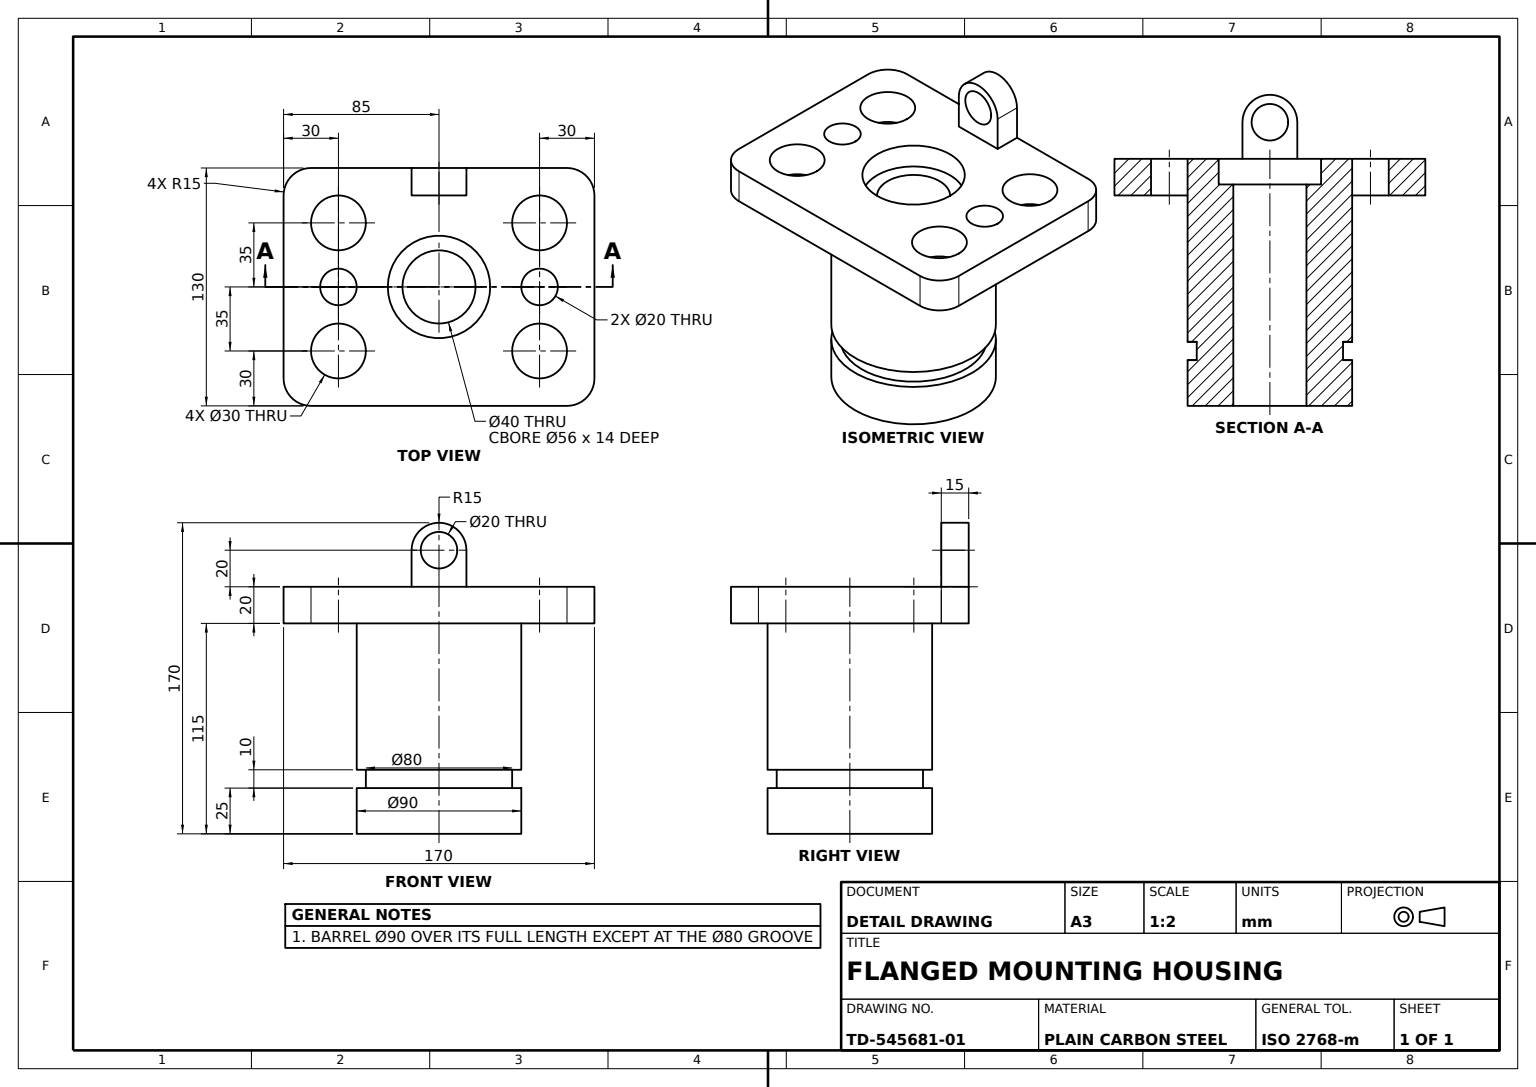
from build123d import *

# Parameters (mm, degrees)
BARREL_SKETCH_R               = 45
HOUSING_BARREL_90_DEPTH       = 115
MOUNTING_FLANGE_SKETCH_W      = 130
MOUNTING_FLANGE_SKETCH_H      = 170
MOUNTING_FLANGE_170X130_DEPTH = 20
FLANGE_HOLES_SKETCH_R         = 15
FLANGE_HOLES_SKETCH_R_2       = 10
FLANGE_MOUNTING_HOLES_DEPTH   = 20
COUNTERBORE_SKETCH_R          = 28
COUNTERBORE_56_DEPTH          = 14
BORE_SKETCH_R                 = 20
BORE_40_DEPTH                 = 162.527087512
BARREL_GROOVE_SKETCH_W        = 45
BARREL_GROOVE_SKETCH_H        = 10
GROOVE_RING_SKETCH_W          = 40
GROOVE_RING_SKETCH_H          = 10
LIFTING_LUG_DEPTH             = 15
LUG_HOLE_SKETCH_R             = 10
LUG_HOLE_20_DEPTH             = 15
FLANGE_CORNER_FILLETS_R15_R   = 15
BOTTOM_RECESS_SKETCH_R        = 20
BOTTOM_RECESS_40_DEPTH        = 15


with BuildPart() as part:
    # Barrel Sketch → Housing Barrel Ø90 (new body)
    with BuildSketch(Plane(origin=(0, 0, 0), x_dir=(1, 0, 0), z_dir=(0, 1, 0))):
        with Locations(Location((0, 0, 0), (0, 0, 270))):
            Circle(BARREL_SKETCH_R)
    extrude(amount=HOUSING_BARREL_90_DEPTH)

    # Mounting Flange Sketch → Mounting Flange 170x130 (add)
    with BuildSketch(Plane(origin=(0, 115, 0), x_dir=(1, 0, 0), z_dir=(0, 1, 0))):
        Rectangle(MOUNTING_FLANGE_SKETCH_W, MOUNTING_FLANGE_SKETCH_H)
    extrude(amount=MOUNTING_FLANGE_170X130_DEPTH)

    # Flange Holes Sketch → Flange Mounting Holes (cut)
    with BuildSketch(Plane(origin=(0, 135, 0), x_dir=(1, 0, 0), z_dir=(0, 1, 0))):
        with Locations(Location((35, 55, 0), (0, 0, 270))):
            Circle(FLANGE_HOLES_SKETCH_R)
        with Locations(Location((0, 55, 0), (0, 0, 270))):
            Circle(FLANGE_HOLES_SKETCH_R_2)
        with Locations(Location((-35, 55, 0), (0, 0, 270))):
            Circle(FLANGE_HOLES_SKETCH_R)
        with Locations(Location((-35, -55, 0), (0, 0, 90))):
            Circle(FLANGE_HOLES_SKETCH_R)
        with Locations(Location((0, -55, 0), (0, 0, 89.999768226))):
            Circle(FLANGE_HOLES_SKETCH_R_2)
        with Locations(Location((35, -55, 0), (0, 0, 90))):
            Circle(FLANGE_HOLES_SKETCH_R)
    extrude(amount=-FLANGE_MOUNTING_HOLES_DEPTH, mode=Mode.SUBTRACT)

    # Counterbore Sketch → Counterbore Ø56 (cut)
    with BuildSketch(Plane(origin=(0, 135, 0), x_dir=(1, 0, 0), z_dir=(0, 1, 0))):
        with Locations(Location((0, 0, 0), (0, 0, 270))):
            Circle(COUNTERBORE_SKETCH_R)
    extrude(amount=-COUNTERBORE_56_DEPTH, mode=Mode.SUBTRACT)

    # Bore Sketch → Bore Ø40 (cut, through all)
    with BuildSketch(Plane(origin=(0, 121, 0), x_dir=(1, 0, 0), z_dir=(0, 1, 0))):
        with Locations(Location((0, 0, 0), (0, 0, 270))):
            Circle(BORE_SKETCH_R)
    extrude(amount=-BORE_40_DEPTH, mode=Mode.SUBTRACT)

    # Barrel Groove Sketch → Barrel Groove (revolve, cut)
    with BuildSketch(Plane.XY, mode=Mode.PRIVATE) as barrel_groove_sk:
        with Locations((-22.5, 30)):
            Rectangle(BARREL_GROOVE_SKETCH_W, BARREL_GROOVE_SKETCH_H)
    revolve(barrel_groove_sk.sketch.rotate(Axis((0, 25, 0), (0, 1, 0)), 90), axis=Axis((0, 25, 0), (0, 1, 0)), mode=Mode.SUBTRACT)


with BuildPart() as barrel_groove_piece_1:
    # of the separate pieces the step leaves, piece 1, a body of its own (barrel_groove_pieces)
    add(part.part.solids().sort_by_distance((-65, 115, 85))[0])



with BuildPart() as barrel_groove_piece_2:
    # of the separate pieces the step leaves, piece 2, a body of its own (barrel_groove_pieces)
    add(part.part.solids().sort_by_distance((0, 0, 45))[0])


with BuildPart() as barrel_groove_piece_1_1:
    add(barrel_groove_piece_1.part)

    add(barrel_groove_piece_2.part)  # Groove Ring merges Barrel Groove piece 2
    # Groove Ring Sketch → Groove Ring (revolve)
    with BuildSketch(Plane.XY, mode=Mode.PRIVATE) as groove_ring_sk:
        with Locations((-20, 30)):
            Rectangle(GROOVE_RING_SKETCH_W, GROOVE_RING_SKETCH_H)
    revolve(groove_ring_sk.sketch.rotate(Axis((0, 25, 0), (0, 1, 0)), 180), axis=Axis((0, 25, 0), (0, 1, 0)))

    # Lifting Lug Sketch → Lifting Lug (add)
    with BuildSketch(Plane.ZY.offset(65)):
        with BuildLine():
            Line((-15, 155), (-15, 135))
            Line((-15, 135), (15, 135))
            Line((15, 135), (15, 155))
            ThreePointArc((15, 155), (0, 170), (-15, 155))
        make_face()
    extrude(amount=-LIFTING_LUG_DEPTH)

    # Lug Hole Sketch → Lug Hole Ø20 (cut)
    with BuildSketch(Plane.ZY.offset(65)):
        with Locations((0, 155)):
            Circle(LUG_HOLE_SKETCH_R)
    extrude(amount=-LUG_HOLE_20_DEPTH, mode=Mode.SUBTRACT)

    # Flange Corner Fillets R15
    flange_corner_fillets_r15_edges = [barrel_groove_piece_1_1.edges().sort_by_distance(p)[0] for p in [
        (65, 125, 85),
        (65, 125, -85),
        (-65, 125, -85),
        (-65, 125, 85),
    ]]
    fillet(flange_corner_fillets_r15_edges, radius=FLANGE_CORNER_FILLETS_R15_R)

    # Bottom Recess Sketch → Bottom Recess Ø40 (cut)
    with BuildSketch(Plane.XZ.offset(-25)):
        with Locations(Location((0, 0, 0), (0, 0, 90))):
            Circle(BOTTOM_RECESS_SKETCH_R)
    extrude(amount=-BOTTOM_RECESS_40_DEPTH, mode=Mode.SUBTRACT)


solid = barrel_groove_piece_1_1.part
